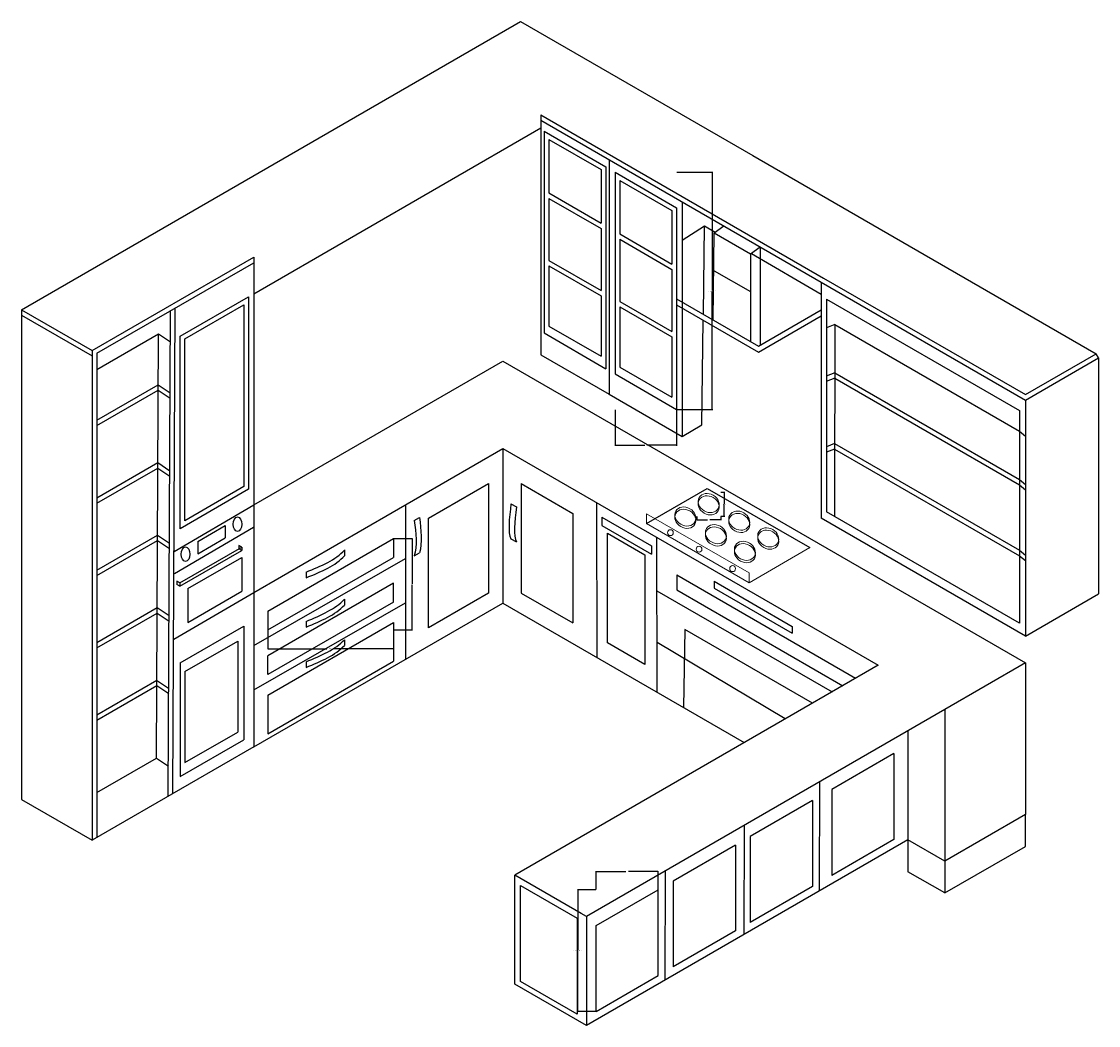
# Model space of a CAD drawing. Units: centimetres. Extents: x 13 to 475, y -355 to 76.
import ezdxf

# ---------------------------------------------------------------- set-up
doc = ezdxf.new("R2010")
doc.units = ezdxf.units.CM
doc.header["$MEASUREMENT"] = 0
for name, color, linetype, lineweight in [('A-ANNO-DIMS', 2, 'Continuous', 18), ('A-EQPM', 8, 'Continuous', 18), ('A-FURN', 7, 'Continuous', 25)]:
    doc.layers.add(name, color=color, linetype=linetype, lineweight=lineweight)
doc.styles.get("Standard").update_dxf_attribs({"font": 'arial.ttf'})
doc.dimstyles.get("Standard").update_dxf_attribs({"dimtxt": 0.18, "dimasz": 0.18, "dimexe": 0.18, "dimexo": 0.0625, "dimgap": 0.09, "dimtad": 0, "dimtih": 1, "dimtoh": 1, "dimdec": 0, "dimzin": 0, "dimdsep": 46, "dimtxsty": 'Standard', "dimcen": 0.09, "dimadec": 0, "dimazin": 0, "dimtfac": 1, "dimtdec": 0, "dimtofl": 0, "dimtmove": 0, "dimatfit": 3, "dimfxl": 1, "dimtolj": 1, "dimtzin": 0, "dimarcsym": 0})

# ---------------------------------------------------------------- blocks, each defined once
blk = doc.blocks.new('BURNER')
for centre in [(4.52, 5.1), (4.52, 4.1)]:
    blk.add_ellipse(centre, major_axis=(-4.08, 2.35), ratio=0.823251)
blk = doc.blocks.new('CAB-DOOR-PANEL')
for p, q in [((0, 36.83), (26.69, 52.24)), ((26.69, 15.41), (26.69, 52.24)), ((0, 0), (0, 36.83)), ((0, 0), (26.69, 15.41))]:
    blk.add_line(p, q)
blk = doc.blocks.new('CAB-GLASS-DOOR')
for p, q in [((0, 101.8), (26.35, 86.59)), ((0, 101.8), (0, 15.33)), ((2, 98.34), (24.35, 85.43)), ((2, 98.34), (2, 75.36)), ((24.35, 85.43), (24.35, 62.46)), ((26.35, 86.59), (26.35, 0)), ((2, 75.36), (24.35, 62.46)), ((2, 73.05), (24.35, 60.15)), ((2, 73.05), (2, 46.42)), ((24.35, 60.15), (24.35, 33.51)), ((2, 46.42), (24.35, 33.51)), ((2, 44.11), (24.35, 31.2)), ((2, 44.11), (2, 18.27)), ((24.35, 31.2), (24.35, 5.37)), ((0, 15.33), (26.35, 0)), ((2, 18.27), (24.35, 5.37))]:
    blk.add_line(p, q)
blk = doc.blocks.new('DRAWER-FRONT')
for p, q in [((0, 8.08), (53.9, 39.2)), ((53.9, 39.2), (53.9, 31.12)), ((0, 0), (53.9, 31.12)), ((0, 8.08), (0, 0))]:
    blk.add_line(p, q)
blk = doc.blocks.new('*D5')
at = {"layer": 'A-ANNO-DIMS', "color": 0, "lineweight": -2, "transparency": 16777216}
for p, q in [((313.26, -126), (314.93, -126)), ((314.75, -126.18), (314.75, -130.98)), ((314.75, -136.14), (314.75, -131.34)), ((313.26, -136.32), (314.93, -136.32))]:
    blk.add_line(p, q, dxfattribs=at)
at = {"layer": 'A-ANNO-DIMS', "color": 0, "transparency": 16777216}
for points in [[(314.72, -126.18), (314.78, -126.18), (314.75, -126)], [(314.72, -136.14), (314.78, -136.14), (314.75, -136.32)]]:
    blk.add_solid(points, dxfattribs=at)
at = {"layer": 'Defpoints', "color": 0, "transparency": 16777216}
for p in [(313.2, -126), (314.75, -126), (313.2, -136.32)]:
    blk.add_point(p, dxfattribs=at)
at = {"layer": 'A-ANNO-DIMS', "color": 0, "transparency": 16777216, "insert": (314.75, -131.16), "char_height": 0.18, "attachment_point": 5}
blk.add_mtext('\\A1;BURNER 10 TYP.', dxfattribs=at)
blk = doc.blocks.new('*D6')
at = {"layer": 'A-ANNO-DIMS', "color": 0, "lineweight": -2, "transparency": 16777216}
for p, q in [((302.91, -136.38), (302.91, -138.05)), ((303.09, -137.87), (307.53, -137.87)), ((313.02, -137.87), (308.57, -137.87)), ((313.2, -136.38), (313.2, -138.05))]:
    blk.add_line(p, q, dxfattribs=at)
at = {"layer": 'A-ANNO-DIMS', "color": 0, "transparency": 16777216}
for points in [[(303.09, -137.84), (303.09, -137.9), (302.91, -137.87)], [(313.02, -137.84), (313.02, -137.9), (313.2, -137.87)]]:
    blk.add_solid(points, dxfattribs=at)
at = {"layer": 'Defpoints', "color": 0, "transparency": 16777216}
for p in [(302.91, -136.32), (313.2, -136.32), (313.2, -137.87)]:
    blk.add_point(p, dxfattribs=at)
at = {"layer": 'A-ANNO-DIMS', "color": 0, "transparency": 16777216, "insert": (308.05, -137.87), "char_height": 0.18, "attachment_point": 5}
blk.add_mtext('\\A1;10 TYP.', dxfattribs=at)
blk = doc.blocks.new('*D7')
at = {"layer": 'A-ANNO-DIMS', "color": 0, "lineweight": -2, "transparency": 16777216}
for p, q in [((259.66, -296.49), (251.71, -296.49)), ((251.89, -296.67), (251.89, -322.43)), ((251.89, -348.55), (251.89, -322.79)), ((259.66, -348.73), (251.71, -348.73))]:
    blk.add_line(p, q, dxfattribs=at)
at = {"layer": 'A-ANNO-DIMS', "color": 0, "transparency": 16777216}
for points in [[(251.86, -296.67), (251.92, -296.67), (251.89, -296.49)], [(251.86, -348.55), (251.92, -348.55), (251.89, -348.73)]]:
    blk.add_solid(points, dxfattribs=at)
at = {"layer": 'Defpoints', "color": 0, "transparency": 16777216}
for p in [(251.89, -296.49), (259.72, -296.49), (259.72, -348.73)]:
    blk.add_point(p, dxfattribs=at)
at = {"layer": 'A-ANNO-DIMS', "color": 0, "transparency": 16777216, "insert": (251.89, -322.61), "char_height": 0.18, "attachment_point": 5}
blk.add_mtext('\\A1;CABINET DOOR PANEL 52 TYP.', dxfattribs=at)
blk = doc.blocks.new('*D8')
at = {"layer": 'A-ANNO-DIMS', "color": 0, "lineweight": -2, "transparency": 16777216}
for p, q in [((259.72, -296.43), (259.72, -288.47)), ((259.9, -288.65), (272.54, -288.65)), ((286.23, -288.65), (273.6, -288.65)), ((286.41, -296.43), (286.41, -288.47))]:
    blk.add_line(p, q, dxfattribs=at)
at = {"layer": 'A-ANNO-DIMS', "color": 0, "transparency": 16777216}
for points in [[(259.9, -288.62), (259.9, -288.68), (259.72, -288.65)], [(286.23, -288.62), (286.23, -288.68), (286.41, -288.65)]]:
    blk.add_solid(points, dxfattribs=at)
at = {"layer": 'Defpoints', "color": 0, "transparency": 16777216}
for p in [(286.41, -288.65), (259.72, -296.49), (286.41, -296.49)]:
    blk.add_point(p, dxfattribs=at)
at = {"layer": 'A-ANNO-DIMS', "color": 0, "transparency": 16777216, "insert": (273.07, -288.65), "char_height": 0.18, "attachment_point": 5}
blk.add_mtext('\\A1;27 TYP.', dxfattribs=at)
blk = doc.blocks.new('*D9')
at = {"layer": 'A-ANNO-DIMS', "color": 0, "lineweight": -2, "transparency": 16777216}
for p, q in [((294.37, 11.18), (309.76, 11.18)), ((309.58, 11), (309.58, -39.54)), ((309.58, -90.44), (309.58, -39.91)), ((294.37, -90.62), (309.76, -90.62))]:
    blk.add_line(p, q, dxfattribs=at)
at = {"layer": 'A-ANNO-DIMS', "color": 0, "transparency": 16777216}
for points in [[(309.55, 11), (309.61, 11), (309.58, 11.18)], [(309.55, -90.44), (309.61, -90.44), (309.58, -90.62)]]:
    blk.add_solid(points, dxfattribs=at)
at = {"layer": 'Defpoints', "color": 0, "transparency": 16777216}
for p in [(294.31, 11.18), (309.58, 11.18), (294.31, -90.62)]:
    blk.add_point(p, dxfattribs=at)
at = {"layer": 'A-ANNO-DIMS', "color": 0, "transparency": 16777216, "insert": (309.58, -39.72), "char_height": 0.18, "attachment_point": 5}
blk.add_mtext('\\A1;GLASS CABINET DOOR 102 TYP.', dxfattribs=at)
blk = doc.blocks.new('*D10')
at = {"layer": 'A-ANNO-DIMS', "color": 0, "lineweight": -2, "transparency": 16777216}
for p, q in [((267.96, -90.69), (267.96, -106.07)), ((294.31, -90.69), (294.31, -106.07)), ((268.14, -105.89), (280.61, -105.89)), ((294.13, -105.89), (281.67, -105.89))]:
    blk.add_line(p, q, dxfattribs=at)
at = {"layer": 'A-ANNO-DIMS', "color": 0, "transparency": 16777216}
for points in [[(268.14, -105.86), (268.14, -105.92), (267.96, -105.89)], [(294.13, -105.86), (294.13, -105.92), (294.31, -105.89)]]:
    blk.add_solid(points, dxfattribs=at)
at = {"layer": 'Defpoints', "color": 0, "transparency": 16777216}
for p in [(267.96, -90.62), (294.31, -90.62), (294.31, -105.89)]:
    blk.add_point(p, dxfattribs=at)
at = {"layer": 'A-ANNO-DIMS', "color": 0, "transparency": 16777216, "insert": (281.14, -105.89), "char_height": 0.18, "attachment_point": 5}
blk.add_mtext('\\A1;26 TYP.', dxfattribs=at)
blk = doc.blocks.new('*D11')
at = {"layer": 'A-ANNO-DIMS', "color": 0, "lineweight": -2, "transparency": 16777216}
for p, q in [((118.9, -185.17), (118.9, -193.37)), ((172.8, -185.17), (172.8, -193.37)), ((119.08, -193.19), (144.27, -193.19)), ((172.62, -193.19), (147.44, -193.19))]:
    blk.add_line(p, q, dxfattribs=at)
at = {"layer": 'A-ANNO-DIMS', "color": 0, "transparency": 16777216}
for points in [[(119.08, -193.16), (119.08, -193.22), (118.9, -193.19)], [(172.62, -193.16), (172.62, -193.22), (172.8, -193.19)]]:
    blk.add_solid(points, dxfattribs=at)
at = {"layer": 'Defpoints', "color": 0, "transparency": 16777216}
for p in [(118.9, -185.1), (172.8, -185.1), (172.8, -193.19)]:
    blk.add_point(p, dxfattribs=at)
at = {"layer": 'A-ANNO-DIMS', "color": 0, "transparency": 16777216, "insert": (145.85, -193.19), "char_height": 0.18, "attachment_point": 5}
blk.add_mtext('\\A1;DRAWER FRONT 54 TYP.', dxfattribs=at)
blk = doc.blocks.new('*D12')
at = {"layer": 'A-ANNO-DIMS', "color": 0, "lineweight": -2, "transparency": 16777216}
for p, q in [((172.86, -145.9), (181.07, -145.9)), ((180.89, -146.08), (180.89, -165.32)), ((180.89, -184.92), (180.89, -165.69)), ((172.86, -185.1), (181.07, -185.1))]:
    blk.add_line(p, q, dxfattribs=at)
at = {"layer": 'A-ANNO-DIMS', "color": 0, "transparency": 16777216}
for points in [[(180.86, -146.08), (180.92, -146.08), (180.89, -145.9)], [(180.86, -184.92), (180.92, -184.92), (180.89, -185.1)]]:
    blk.add_solid(points, dxfattribs=at)
at = {"layer": 'Defpoints', "color": 0, "transparency": 16777216}
for p in [(172.8, -145.9), (180.89, -145.9), (172.8, -185.1)]:
    blk.add_point(p, dxfattribs=at)
at = {"layer": 'A-ANNO-DIMS', "color": 0, "transparency": 16777216, "insert": (180.89, -165.5), "char_height": 0.18, "attachment_point": 5}
blk.add_mtext('\\A1;39 TYP.', dxfattribs=at)

msp = doc.modelspace()

# ---------------------------------------------------------------- linework, layer by layer
at = {"layer": 'A-EQPM'}
for p, q in [((281.34, -139.44), (281.34, -135.23)), ((325.34, -160.64), (281.34, -135.23)), ((281.34, -139.44), (325.34, -164.84)), ((325.34, -164.84), (351.44, -149.77)), ((325.34, -164.84), (325.34, -160.64))]:
    msp.add_line(p, q, dxfattribs=at)
for centre in [(291.64, -143.38), (303.9, -150.46), (318.32, -158.79)]:
    msp.add_ellipse(centre, major_axis=(0, 1.27), ratio=0.971238, dxfattribs=at)
at = {"layer": 'A-FURN'}
for p, q in [((13.33, -47.78), (227.4, 75.82)), ((227.4, 75.82), (326.99, 18.32)), ((236.06, 35.82), (296.68, 0.82)), ((236.06, 35.82), (236.06, -67.07)), ((236.06, 33.51), (295.68, -0.92)), ((112.92, -40.9), (236.06, 30.19)), ((265.37, 16.58), (265.37, -83.99)), ((326.99, 18.32), (387.62, -16.68)), ((296.68, 0.82), (357.3, -34.18)), ((295.68, -0.92), (356.3, -35.92)), ((296.68, -1.49), (296.68, -102.07)), ((296.68, -17.88), (306.25, -11.83)), ((305.76, -49.69), (306.25, -11.83)), ((306.25, -11.83), (310.88, -14.54)), ((310.44, -14.86), (314.6, -11.84)), ((309.96, -52.12), (310.44, -14.86)), ((310.44, -14.86), (326.04, -23.86)), ((387.62, -16.68), (474.22, -66.68)), ((326.04, -23.86), (330.19, -20.84)), ((330.19, -20.84), (330.08, -63.02)), ((43.64, -65.28), (112.92, -25.28)), ((45.64, -66.43), (112.92, -27.59)), ((112.92, -25.28), (112.92, -235.28)), ((326.04, -23.86), (325.94, -61.34)), ((326.39, -23.6), (356.3, -41.09)), ((310.4, -31.02), (325.99, -40.02)), ((356.3, -35.92), (443.91, -86.49)), ((356.3, -35.92), (356.3, -137.12)), ((357.3, -34.18), (443.91, -84.18)), ((81.38, -59.12), (110.74, -42.17)), ((83.38, -60.27), (108.74, -45.63)), ((108.74, -45.63), (108.74, -123.62)), ((110.74, -42.17), (110.74, -124.78)), ((294.31, -43.08), (329.47, -63.38)), ((294.31, -45.63), (329.47, -65.92)), ((358.55, -43.17), (358.55, -134.39)), ((358.55, -43.17), (441.33, -90.96)), ((13.33, -47.78), (13.33, -257.78)), ((13.33, -47.78), (43.64, -65.28)), ((13.33, -50.09), (43.64, -67.59)), ((76.28, -256.43), (77.28, -48.17)), ((78.28, -255.28), (79.28, -47.01)), ((329.47, -63.38), (356.3, -47.88)), ((329.47, -65.92), (356.3, -50.43)), ((305.15, -97.18), (305.73, -52.22)), ((362.16, -54.13), (358.55, -55.51)), ((362.16, -54.13), (362.11, -77.18)), ((362.16, -54.13), (441.33, -99.84)), ((45.64, -73.33), (72.02, -58.1)), ((71.15, -240.02), (72.02, -58.1)), ((72.01, -58.1), (77.2, -61.53)), ((81.38, -141.72), (81.38, -59.12)), ((83.38, -138.26), (83.38, -60.27)), ((43.64, -65.28), (43.64, -275.28)), ((45.64, -66.43), (45.64, -274.12)), ((236.06, -67.07), (265.37, -83.99)), ((443.91, -84.18), (474.22, -66.68)), ((443.91, -86.49), (475.22, -68.42)), ((475.22, -68.42), (474.22, -66.68)), ((475.22, -68.42), (475.22, -169.62)), ((112.92, -131.48), (219.77, -69.8)), ((219.77, -69.8), (443.91, -199.21)), ((362.11, -74.88), (358.5, -76.25)), ((362.11, -77.18), (358.5, -78.56)), ((362.11, -77.18), (362.04, -107.5)), ((362.11, -74.88), (441.33, -120.58)), ((362.11, -77.18), (441.33, -122.89)), ((45.64, -95.12), (71.91, -79.95)), ((45.64, -97.43), (71.9, -82.27)), ((71.9, -82.27), (77.1, -85.7)), ((71.91, -79.95), (77.11, -83.38)), ((265.37, -83.99), (296.68, -102.07)), ((443.91, -86.49), (443.91, -187.7)), ((441.33, -90.96), (441.33, -182.19)), ((296.68, -102.07), (305.15, -97.18)), ((441.33, -99.84), (443.91, -101.97)), ((362.05, -105.19), (358.55, -106.52)), ((362.05, -105.19), (441.33, -150.93)), ((112.92, -168.96), (219.77, -107.27)), ((219.77, -107.27), (380.74, -200.21)), ((219.77, -107.27), (219.77, -173.59)), ((362.04, -107.5), (358.55, -108.83)), ((362.04, -107.5), (361.98, -136.38)), ((362.04, -107.5), (441.33, -153.24)), ((45.64, -128.43), (71.75, -113.35)), ((71.75, -113.35), (76.95, -116.79)), ((45.64, -130.74), (71.74, -115.67)), ((71.74, -115.67), (76.94, -119.1)), ((108.74, -123.62), (83.38, -138.26)), ((187.83, -137.22), (213.62, -122.34)), ((213.62, -122.34), (213.62, -169.33)), ((227.68, -122.34), (227.68, -169.33)), ((227.68, -122.34), (249.78, -135.1)), ((281.34, -139.44), (307.44, -124.37)), ((307.44, -124.37), (351.44, -149.77)), ((441.33, -120.58), (443.91, -122.71)), ((441.33, -122.89), (443.91, -125.02)), ((110.74, -124.78), (81.38, -141.72)), ((78.78, -151.45), (112.92, -131.48)), ((178.01, -131.38), (178.01, -197.7)), ((223.24, -131), (225.57, -132.35)), ((260.16, -196.91), (260.06, -130.54)), ((181.77, -138.09), (183.99, -136.81)), ((187.83, -184.22), (187.83, -137.22)), ((249.78, -135.1), (249.78, -182.09)), ((262.28, -136.79), (283.59, -149.09)), ((262.28, -136.79), (262.28, -140.26)), ((443.91, -187.7), (356.3, -137.12)), ((441.33, -182.19), (358.55, -134.39)), ((78.87, -160.84), (112.88, -140.95)), ((88.93, -147.11), (100.67, -140.33)), ((100.67, -140.33), (100.67, -145.65)), ((262.28, -140.26), (283.59, -152.56)), ((45.64, -159.43), (71.61, -144.44)), ((45.64, -161.74), (71.59, -146.76)), ((71.59, -144.44), (76.79, -147.87)), ((71.59, -146.76), (76.79, -150.19)), ((88.93, -152.43), (100.67, -145.65)), ((88.93, -147.11), (88.93, -152.43)), ((223.24, -146), (225.57, -147.35)), ((264.6, -190.65), (264.6, -143.65)), ((264.6, -143.65), (280.69, -152.94)), ((285.93, -211.79), (285.84, -145.42)), ((81.24, -164.88), (107.81, -149.54)), ((81.24, -166.37), (107.81, -151.02)), ((106.12, -150.52), (106.11, -150.52)), ((106.11, -150.52), (106.11, -150.52)), ((106.11, -150.52), (106.12, -150.52)), ((107.81, -149.54), (106.58, -148.83)), ((106.58, -148.83), (106.58, -150.31)), ((107.81, -151.02), (106.58, -150.31)), ((107.81, -149.54), (107.81, -151.02)), ((151.79, -150.8), (151.79, -153.26)), ((181.77, -153.37), (183.99, -152.09)), ((283.59, -149.09), (283.59, -152.56)), ((441.33, -150.93), (443.91, -153.06)), ((84.69, -167.31), (107.81, -153.96)), ((103.6, -153.46), (103.59, -153.46)), ((103.6, -153.46), (103.59, -153.46)), ((107.81, -153.96), (107.81, -168.5)), ((112.92, -191.82), (178.01, -154.43)), ((280.69, -152.94), (280.69, -199.94)), ((441.33, -153.24), (443.91, -155.37)), ((135.41, -160.25), (135.41, -162.72)), ((294.43, -161.5), (371.03, -205.82)), ((294.43, -161.5), (294.43, -167.88)), ((81.24, -164.88), (80, -164.17)), ((80, -164.17), (80, -165.65)), ((81.24, -166.37), (80, -165.65)), ((81.24, -164.88), (81.24, -166.37)), ((310.4, -164.24), (343.91, -183.59)), ((310.4, -164.24), (310.4, -167.2)), ((78.6, -189.03), (112.92, -168.96)), ((84.69, -167.31), (84.69, -181.85)), ((84.69, -181.85), (107.81, -168.5)), ((213.62, -169.33), (187.83, -184.22)), ((227.68, -169.33), (249.78, -182.09)), ((285.87, -168.27), (361.01, -211.61)), ((294.43, -167.88), (365.52, -209)), ((310.4, -167.2), (343.91, -186.54)), ((443.91, -187.7), (475.22, -169.62)), ((112.92, -210.81), (178.01, -173.42)), ((112.92, -235.28), (219.77, -173.59)), ((151.79, -171.96), (151.79, -174.43)), ((219.77, -173.59), (323.31, -233.37)), ((45.64, -190.43), (71.46, -175.53)), ((45.64, -192.74), (71.44, -177.84)), ((71.44, -177.84), (76.64, -181.28)), ((71.46, -175.53), (76.65, -178.96)), ((81.38, -199.23), (108.74, -183.43)), ((108.74, -183.43), (108.74, -232.21)), ((118.9, -213.03), (172.8, -181.91)), ((135.41, -181.42), (135.41, -183.88)), ((172.8, -181.91), (172.8, -198.5)), ((343.91, -183.59), (343.91, -186.54)), ((151.79, -189.27), (151.79, -191.73)), ((151.79, -189.27), (151.79, -191.73)), ((297.88, -184.9), (297.21, -218.3)), ((352.57, -216.48), (297.88, -184.9)), ((83.38, -202.94), (106.08, -189.83)), ((106.08, -189.83), (106.08, -228.88)), ((280.69, -199.94), (264.6, -190.65)), ((340.91, -223.21), (285.9, -190.47)), ((118.9, -229.62), (172.8, -198.5)), ((81.38, -199.23), (81.38, -248)), ((83.38, -202.94), (83.38, -241.98)), ((135.41, -198.72), (135.41, -201.18)), ((135.41, -198.72), (135.41, -201.18)), ((380.74, -200.21), (346.1, -220.21)), ((443.91, -199.21), (409.27, -219.21)), ((443.91, -199.21), (443.91, -264.21)), ((45.64, -221.43), (71.31, -206.61)), ((71.23, -206.66), (76.42, -210.09)), ((45.64, -223.74), (71.3, -208.93)), ((71.3, -208.93), (76.49, -212.36)), ((118.9, -213.03), (118.9, -229.62)), ((346.1, -220.21), (224.86, -290.21)), ((409.27, -219.21), (255.57, -307.94)), ((409.27, -219.21), (409.27, -284.21)), ((83.38, -241.98), (106.08, -228.88)), ((393.47, -228.33), (393.47, -288.76)), ((112.92, -235.28), (43.64, -275.28)), ((81.38, -248), (108.74, -232.21)), ((45.64, -254.74), (71.15, -240.02)), ((71.15, -240.02), (76.34, -243.45)), ((355.6, -250.19), (355.42, -297.05)), ((13.33, -257.78), (43.64, -275.28)), ((443.91, -264.21), (409.27, -284.21)), ((443.91, -277.89), (443.91, -264.21)), ((323.33, -268.82), (323.15, -315.69)), ((393.47, -275.09), (255.57, -354.7)), ((409.27, -284.21), (393.47, -275.09)), ((409.27, -297.89), (443.91, -277.89)), ((409.27, -284.21), (409.27, -297.89)), ((224.86, -336.97), (224.86, -290.21)), ((253.38, -306.68), (224.86, -290.21)), ((289.4, -288.41), (289.22, -335.27)), ((409.27, -297.89), (393.47, -288.76)), ((227.38, -294.66), (251.62, -308.66)), ((227.38, -335.82), (227.38, -294.66)), ((251.62, -308.66), (251.62, -349.82)), ((255.57, -307.94), (253.38, -306.68)), ((255.57, -307.94), (255.57, -354.7)), ((255.57, -354.7), (224.86, -336.97)), ((251.62, -349.82), (227.38, -335.82))]:
    msp.add_line(p, q, dxfattribs=at)
for centre in [(105.98, -139.75), (83.71, -152.61)]:
    msp.add_ellipse(centre, major_axis=(0, 3.1), ratio=0.596565, dxfattribs=at)
for points in [[(223.24, -131), (222.52, -137.26), (221.79, -143.52), (223.24, -146)], [(225.57, -132.35), (224.85, -138.6), (224.12, -144.86), (225.57, -147.35)], [(181.77, -138.09), (182.44, -143.57), (183.12, -149.06), (181.77, -153.37)], [(183.99, -136.81), (184.66, -142.29), (185.34, -147.77), (183.99, -152.09)], [(135.41, -160.25), (141.8, -157.65), (148.19, -155.05), (151.79, -150.84)], [(135.41, -162.72), (141.8, -160.11), (148.19, -157.51), (151.79, -153.3)], [(135.41, -181.42), (141.73, -178.76), (148.05, -176.11), (151.79, -171.96)], [(135.41, -183.88), (141.73, -181.23), (148.05, -178.57), (151.79, -174.43)], [(135.41, -198.72), (141.73, -196.07), (148.05, -193.41), (151.79, -189.27)], [(135.41, -201.18), (141.73, -198.53), (148.05, -195.88), (151.79, -191.73)]]:
    msp.add_open_spline(points, degree=3, dxfattribs=at)

# ---------------------------------------------------------------- block references
at = {"layer": 'A-EQPM'}
for p in [(303.54, -135.76), (293.52, -141.54), (316.62, -143.31), (306.6, -149.1), (329.06, -150.5), (319.04, -156.28)]:
    msp.add_blockref('BURNER', p, dxfattribs=at)
at = {"layer": 'A-FURN'}
for name, p in [('CAB-GLASS-DOOR', (237.55, -73.06)), ('CAB-GLASS-DOOR', (267.96, -90.62)), ('DRAWER-FRONT', (118.9, -185.1)), ('CAB-DOOR-PANEL', (259.72, -348.73))]:
    msp.add_blockref(name, p, dxfattribs=at)
at = {"layer": 'A-FURN', "rotation": 180}
for name, p in [('DRAWER-FRONT', (172.8, -165.06)), ('CAB-DOOR-PANEL', (387.5, -238.13)), ('CAB-DOOR-PANEL', (352.56, -258.3)), ('CAB-DOOR-PANEL', (319.57, -277.35))]:
    msp.add_blockref(name, p, dxfattribs=at)

# ---------------------------------------------------------------- dimensions: what is measured, and where the dimension line sits
at = {"layer": 'A-ANNO-DIMS'}
for base, p1, p2, text, picture, middle in [((309.58, 11.18), (294.31, -90.62), (294.31, 11.18), 'GLASS CABINET DOOR <> TYP.', '*D9', (309.58, -39.72)), ((314.75, -126), (313.2, -136.32), (313.2, -126), 'BURNER <> TYP.', '*D5', (314.75, -131.16)), ((180.89, -145.9), (172.8, -185.1), (172.8, -145.9), '<> TYP.', '*D12', (180.89, -165.5)), ((251.89, -296.49), (259.72, -348.73), (259.72, -296.49), 'CABINET DOOR PANEL <> TYP.', '*D7', (251.89, -322.61))]:
    dim = msp.add_linear_dim(base=base, p1=p1, p2=p2, angle=90, text=text, dimstyle='Standard', override={"dimdec": 0, "dimlfac": 1, "dimrnd": 0, "dimzin": 0, "dimdsep": 46, "dimlunit": 2}, dxfattribs=at)
    dim.commit()
    dim.dimension.update_dxf_attribs({"geometry": picture, "text_midpoint": middle})
for base, p1, p2, text, picture, middle in [((294.31, -105.89), (267.96, -90.62), (294.31, -90.62), '<> TYP.', '*D10', (281.14, -105.89)), ((313.2, -137.87), (302.91, -136.32), (313.2, -136.32), '<> TYP.', '*D6', (308.05, -137.87)), ((172.8, -193.19), (118.9, -185.1), (172.8, -185.1), 'DRAWER FRONT <> TYP.', '*D11', (145.85, -193.19)), ((286.41, -288.65), (259.72, -296.49), (286.41, -296.49), '<> TYP.', '*D8', (273.07, -288.65))]:
    dim = msp.add_linear_dim(base=base, p1=p1, p2=p2, text=text, dimstyle='Standard', override={"dimdec": 0, "dimlfac": 1, "dimrnd": 0, "dimzin": 0, "dimdsep": 46, "dimlunit": 2}, dxfattribs=at)
    dim.commit()
    dim.dimension.update_dxf_attribs({"geometry": picture, "text_midpoint": middle})

doc.saveas('drawing.dxf')
